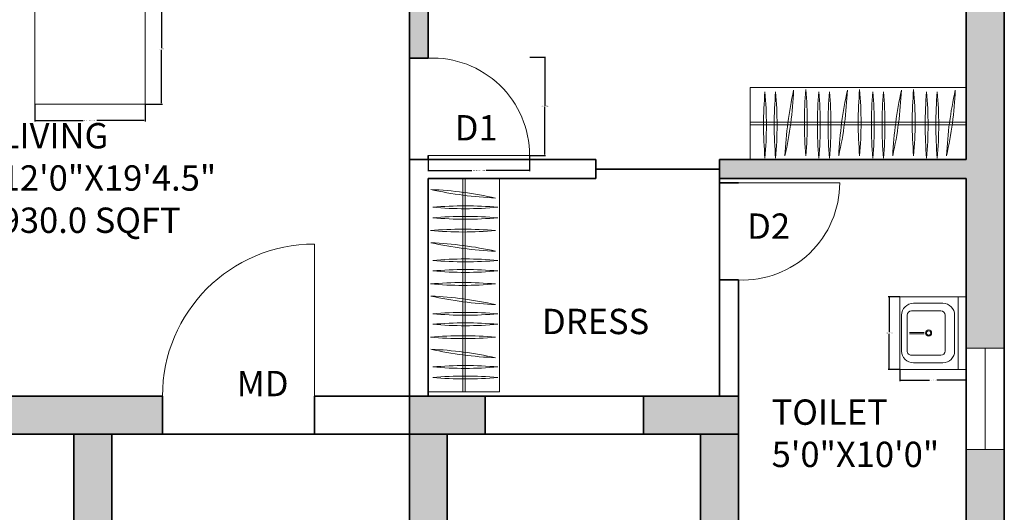
# Model space of a CAD drawing. Units: inches. Extents: x -9 to 505, y -680 to 48.
# Tile 7 of 17: x 235 to 469, y -314 to -198. Entities that reach past the tile are written whole.
import ezdxf

# ---------------------------------------------------------------- set-up
doc = ezdxf.new("R2010")
doc.units = ezdxf.units.IN
doc.header["$MEASUREMENT"] = 0
for name, color, linetype, lineweight in [('A-ANNO-DIMS', 2, 'Continuous', 18), ('A-ANNO-TEXT', 7, 'Continuous', 18), ('A-AREA-IDEN', 7, 'Continuous', 18), ('A-DOOR', 3, 'Continuous', 18), ('A-FLOR-CASE', 8, 'Continuous', 18), ('A-FLOR-FIXT', 9, 'Continuous', 18), ('A-FURN', 8, 'Continuous', 18), ('A-GLAZ', 4, 'Continuous', 18), ('A-WALL', 7, 'Continuous', 35), ('A-WALL-PATT', 251, 'Continuous', 13), ('S-CONC', 7, 'Continuous', 35), ('S-CONC-PATT', 18, 'Continuous', 13)]:
    doc.layers.add(name, color=color, linetype=linetype, lineweight=lineweight)
doc.styles.get("Standard").update_dxf_attribs({"font": 'arial.ttf'})
doc.dimstyles.get("Standard").update_dxf_attribs({"dimtxt": 0.18, "dimasz": 0.18, "dimexe": 0.18, "dimexo": 0.0625, "dimgap": 0.09, "dimtad": 0, "dimtih": 1, "dimtoh": 1, "dimdec": 0, "dimzin": 0, "dimdsep": 46, "dimlunit": 3, "dimtxsty": 'Standard', "dimcen": 0.09, "dimadec": 0, "dimazin": 0, "dimtfac": 1, "dimtdec": 0, "dimtofl": 0, "dimtmove": 0, "dimatfit": 3, "dimfxl": 1, "dimtolj": 1, "dimtzin": 0, "dimarcsym": 0})

# ---------------------------------------------------------------- blocks, each defined once
blk = doc.blocks.new('М14 600х655')
for p, q in [((-655, 600), (-655, 0)), ((-655, 600), (-655, 0)), ((-655, 0), (-655, 600)), ((0, 600), (-655, 600)), ((0, 0), (0, 600)), ((0, 525), (-655, 525)), ((-165.1, 494.1), (-489.9, 494.1)), ((-595.8, 388.1), (-595.8, 121.3)), ((-528.4, 370.1), (-528.4, 103.3)), ((-165.4, 408.4), (-490.2, 408.4)), ((-127.2, 103.3), (-127.2, 370.1)), ((-59.2, 121.3), (-59.2, 388.1)), ((-333.5, 87.1), (-333.5, 219.6)), ((-321.5, 87.1), (-321.5, 219.6)), ((-655, 0), (-655, 0)), ((-655, 0), (-655, 0)), ((-655, 0), (0, 0)), ((-655, 0), (0, 0)), ((-490.2, 65.1), (-165.4, 65.1)), ((-489.9, 15.4), (-165.1, 15.4))]:
    blk.add_line(p, q)
for radius in [27.6, 19.3]:
    blk.add_circle((-327.5, 258.9), radius)
for centre, radius, start, end in [((-489.9, 388.1), 105.9, 90, 180), ((-165.1, 388.1), 105.9, 0, 90), ((-490.2, 370.1), 38.2, 90, 180), ((-165.4, 370.1), 38.2, 0, 90), ((-489.9, 121.3), 105.9, 180, 270), ((-490.2, 103.3), 38.2, 180, 270), ((-165.4, 103.3), 38.2, 270, 0), ((-165.1, 121.3), 105.9, 270, 0)]:
    blk.add_arc(centre, radius, start, end)
blk = doc.blocks.new('WARDROBE-HANGING')
for p, q in [((51.19, 17.07), (0, 17.07)), ((0, 17.07), (0, 0)), ((51.19, 17.07), (51.19, 0)), ((51.19, 8.82), (0, 8.82)), ((51.19, 8.25), (0, 8.25)), ((51.19, 0), (0, 0))]:
    blk.add_line(p, q)
for centre, start, end in [((-79.45, 20.34), 347.508, 357.5023), ((97.92, -3), 167.508, 177.5023), ((102.6, 8.74), 175.0028, 184.9972), ((-76.3, 8.74), 355.0028, 4.9972), ((-66.7, 20.34), 347.508, 357.5023), ((110.67, -3), 167.508, 177.5023), ((115.36, 8.74), 175.0028, 184.9972), ((-63.54, 8.74), 355.0028, 4.9972), ((123.47, -3), 167.508, 177.5023), ((-53.9, 20.34), 347.508, 357.5023), ((128.16, 8.74), 175.0028, 184.9972), ((-50.74, 8.74), 355.0028, 4.9972), ((136.23, -3), 167.508, 177.5023), ((-41.14, 20.34), 347.508, 357.5023), ((92.92, 8.19), 175.0028, 184.9972), ((-85.98, 8.19), 355.0028, 4.9972), ((95.45, 8.19), 175.0028, 184.9972), ((-83.45, 8.19), 355.0028, 4.9972), ((105.68, 8.19), 175.0028, 184.9972), ((-73.22, 8.19), 355.0028, 4.9972), ((108.21, 8.19), 175.0028, 184.9972), ((-70.69, 8.19), 355.0028, 4.9972), ((118.48, 8.19), 175.0028, 184.9972), ((-60.42, 8.19), 355.0028, 4.9972), ((121.01, 8.19), 175.0028, 184.9972), ((-57.89, 8.19), 355.0028, 4.9972), ((131.23, 8.19), 175.0028, 184.9972), ((-47.67, 8.19), 355.0028, 4.9972), ((133.76, 8.19), 175.0028, 184.9972), ((-45.14, 8.19), 355.0028, 4.9972)]:
    blk.add_arc(centre, 89.79, start, end)
blk = doc.blocks.new('WIN-24')
for p, q in [((0, 24), (0, 0)), ((9, 24), (0, 24)), ((4.5, 24), (4.5, 2.23)), ((9, 0), (9, 24)), ((0, 0), (9, 0)), ((4.5, 2.23), (4.5, 0))]:
    blk.add_line(p, q)
blk = doc.blocks.new('DOOR-SWING-24')
blk.add_line((0, 0), (24, 0))
blk.add_arc((0.98, 0), 23.02, 0, 92.4378)
blk = doc.blocks.new('DOOR-ENTRY-36')
blk.add_line((36, 0), (36, 36))
blk.add_arc((36, 0), 36, 90, 180)
blk = doc.blocks.new('TABLE-COFFEE-SQUARE')
at = {"ltscale": 0.03}
blk.add_lwpolyline([(0, 0), (26.11, 0), (26.11, 26.11), (0, 26.11)], close=True, dxfattribs=at)
blk = doc.blocks.new('*D24')
at = {"layer": 'A-ANNO-DIMS', "color": 0, "lineweight": -2, "transparency": 16777216}
for p, q in [((332.26, -230.06), (332.26, -233.78)), ((356.26, -230.06), (356.26, -233.78)), ((332.44, -233.6), (342.58, -233.6)), ((356.08, -233.6), (345.94, -233.6))]:
    blk.add_line(p, q, dxfattribs=at)
at = {"layer": 'A-ANNO-DIMS', "color": 0, "transparency": 16777216}
for points in [[(332.44, -233.57), (332.44, -233.63), (332.26, -233.6)], [(356.08, -233.57), (356.08, -233.63), (356.26, -233.6)]]:
    blk.add_solid(points, dxfattribs=at)
at = {"layer": 'Defpoints', "color": 0, "transparency": 16777216}
for p in [(332.26, -230), (356.26, -230), (356.26, -233.6)]:
    blk.add_point(p, dxfattribs=at)
at = {"layer": 'A-ANNO-DIMS', "color": 0, "transparency": 16777216, "insert": (344.26, -233.6), "char_height": 0.18, "attachment_point": 5}
blk.add_mtext('\\A1;INTERIOR DOOR 2\'-0" TYP.', dxfattribs=at)
blk = doc.blocks.new('*D25')
at = {"layer": 'A-ANNO-DIMS', "color": 0, "lineweight": -2, "transparency": 16777216}
for p, q in [((356.33, -206.73), (360.04, -206.73)), ((359.86, -206.91), (359.86, -218.18)), ((359.86, -229.82), (359.86, -218.55)), ((356.33, -230), (360.04, -230))]:
    blk.add_line(p, q, dxfattribs=at)
at = {"layer": 'A-ANNO-DIMS', "color": 0, "transparency": 16777216}
for points in [[(359.83, -206.91), (359.89, -206.91), (359.86, -206.73)], [(359.83, -229.82), (359.89, -229.82), (359.86, -230)]]:
    blk.add_solid(points, dxfattribs=at)
at = {"layer": 'Defpoints', "color": 0, "transparency": 16777216}
for p in [(356.26, -206.73), (359.86, -206.73), (356.26, -230)]:
    blk.add_point(p, dxfattribs=at)
at = {"layer": 'A-ANNO-DIMS', "color": 0, "transparency": 16777216, "insert": (359.86, -218.37), "char_height": 0.18, "attachment_point": 5}
blk.add_mtext('\\A1;1\'-11 1/2" TYP.', dxfattribs=at)
blk = doc.blocks.new('*D36')
at = {"layer": 'A-ANNO-DIMS', "color": 0, "lineweight": -2, "transparency": 16777216}
for p, q in [((443.97, -263.48), (441.27, -263.48)), ((441.45, -263.66), (441.45, -271.88)), ((441.45, -280.47), (441.45, -272.25)), ((443.97, -280.65), (441.27, -280.65))]:
    blk.add_line(p, q, dxfattribs=at)
at = {"layer": 'A-ANNO-DIMS', "color": 0, "transparency": 16777216}
for points in [[(441.42, -263.66), (441.48, -263.66), (441.45, -263.48)], [(441.42, -280.47), (441.48, -280.47), (441.45, -280.65)]]:
    blk.add_solid(points, dxfattribs=at)
at = {"layer": 'Defpoints', "color": 0, "transparency": 16777216}
for p in [(444.03, -263.48), (441.45, -280.65), (444.03, -280.65)]:
    blk.add_point(p, dxfattribs=at)
at = {"layer": 'A-ANNO-DIMS', "color": 0, "transparency": 16777216, "insert": (441.45, -272.06), "char_height": 0.18, "attachment_point": 5}
blk.add_mtext('\\A1;BASIN 1\'-5" TYP.', dxfattribs=at)
blk = doc.blocks.new('*D37')
at = {"layer": 'A-ANNO-DIMS', "color": 0, "lineweight": -2, "transparency": 16777216}
for p, q in [((444.03, -280.71), (444.03, -283.41)), ((459.76, -280.71), (459.76, -283.41)), ((444.21, -283.23), (451.06, -283.23)), ((459.58, -283.23), (452.74, -283.23))]:
    blk.add_line(p, q, dxfattribs=at)
at = {"layer": 'A-ANNO-DIMS', "color": 0, "transparency": 16777216}
for points in [[(444.21, -283.2), (444.21, -283.26), (444.03, -283.23)], [(459.58, -283.2), (459.58, -283.26), (459.76, -283.23)]]:
    blk.add_solid(points, dxfattribs=at)
at = {"layer": 'Defpoints', "color": 0, "transparency": 16777216}
for p in [(444.03, -280.65), (459.76, -280.65), (459.76, -283.23)]:
    blk.add_point(p, dxfattribs=at)
at = {"layer": 'A-ANNO-DIMS', "color": 0, "transparency": 16777216, "insert": (451.9, -283.23), "char_height": 0.18, "attachment_point": 5}
blk.add_mtext('\\A1;1\'-3 1/2" TYP.', dxfattribs=at)
blk = doc.blocks.new('*D38')
at = {"layer": 'A-ANNO-DIMS', "color": 0, "lineweight": -2, "transparency": 16777216}
for p, q in [((239.02, -217.94), (239.02, -221.97)), ((265.13, -217.94), (265.13, -221.97)), ((239.2, -221.79), (250.46, -221.79)), ((264.95, -221.79), (253.7, -221.79))]:
    blk.add_line(p, q, dxfattribs=at)
at = {"layer": 'A-ANNO-DIMS', "color": 0, "transparency": 16777216}
for points in [[(239.2, -221.76), (239.2, -221.82), (239.02, -221.79)], [(264.95, -221.76), (264.95, -221.82), (265.13, -221.79)]]:
    blk.add_solid(points, dxfattribs=at)
at = {"layer": 'Defpoints', "color": 0, "transparency": 16777216}
for p in [(239.02, -217.87), (265.13, -217.87), (265.13, -221.79)]:
    blk.add_point(p, dxfattribs=at)
at = {"layer": 'A-ANNO-DIMS', "color": 0, "transparency": 16777216, "insert": (252.08, -221.79), "char_height": 0.18, "attachment_point": 5}
blk.add_mtext('\\A1;COFFEE TABLE 2\'-2" TYP.', dxfattribs=at)
blk = doc.blocks.new('*D39')
at = {"layer": 'A-ANNO-DIMS', "color": 0, "lineweight": -2, "transparency": 16777216}
for p, q in [((265.2, -191.76), (269.23, -191.76)), ((269.05, -191.94), (269.05, -204.64)), ((269.05, -217.69), (269.05, -205)), ((265.2, -217.87), (269.23, -217.87))]:
    blk.add_line(p, q, dxfattribs=at)
at = {"layer": 'A-ANNO-DIMS', "color": 0, "transparency": 16777216}
for points in [[(269.02, -191.94), (269.08, -191.94), (269.05, -191.76)], [(269.02, -217.69), (269.08, -217.69), (269.05, -217.87)]]:
    blk.add_solid(points, dxfattribs=at)
at = {"layer": 'Defpoints', "color": 0, "transparency": 16777216}
for p in [(265.13, -191.76), (269.05, -191.76), (265.13, -217.87)]:
    blk.add_point(p, dxfattribs=at)
at = {"layer": 'A-ANNO-DIMS', "color": 0, "transparency": 16777216, "insert": (269.05, -204.82), "char_height": 0.18, "attachment_point": 5}
blk.add_mtext('\\A1;2\'-2" TYP.', dxfattribs=at)

msp = doc.modelspace()

# ---------------------------------------------------------------- hatches: boundary and pattern name
at = {"layer": 'A-WALL-PATT'}
h = msp.add_hatch(color=256, dxfattribs=at)
h.dxf.hatch_style = 1
h.paths.add_polyline_path([(101.64, 11.5), (48.26, 11.5), (48.26, 2.5), (72.26, 2.5), (72.26, -21.25), (81.26, -21.25), (81.26, 2.5), (101.64, 2.5)])
h.paths.add_polyline_path([(36.26, 2.5), (27.26, 2.5), (27.26, -6.92), (36.26, -6.92)])
h.paths.add_polyline_path([(81.26, -57.25), (72.26, -57.25), (72.26, -75.5), (81.26, -75.5)])
h.paths.add_polyline_path([(162.76, 11.5), (137.64, 11.5), (137.64, 2.5), (162.76, 2.5)])
h.paths.add_polyline_path([(179.26, 2.5), (174.76, 2.5), (174.76, -75.5), (179.26, -75.5), (179.26, -54.5), (229.51, -54.5), (229.51, -45.5), (179.26, -45.5)])
h.paths.add_polyline_path([(382.26, -45.5), (332.26, -45.5), (332.26, 2.5), (327.76, 2.5), (327.76, -45.5), (277.51, -45.5), (277.51, -54.5), (327.76, -54.5), (327.76, -111.5), (332.26, -111.5), (332.26, -54.5), (382.26, -54.5)])
h.paths.add_polyline_path([(332.26, -128), (327.76, -128), (327.76, -207), (332.26, -207)])
h.paths.add_polyline_path([(124.76, -111.5), (36.26, -111.5), (36.26, -116), (120.26, -116), (120.26, -168.5), (179.26, -168.5), (179.26, -164), (124.76, -164)])
h.paths.add_polyline_path([(96.26, -164), (36.26, -164), (36.26, -152), (27.26, -152), (27.26, -208.88), (36.26, -208.88), (36.26, -168.5), (96.26, -168.5)])
h.paths.add_polyline_path([(36.26, -244.88), (27.26, -244.88), (27.26, -287), (36.26, -287)])
h.paths.add_polyline_path([(179.26, -204.5), (174.76, -204.5), (174.76, -287), (179.26, -287)])
h.paths.add_polyline_path([(257.26, -296), (248.26, -296), (248.26, -446), (269.26, -446), (269.26, -437), (257.26, -437)])
h.paths.add_polyline_path([(90.26, -296), (81.26, -296), (81.26, -348.67), (90.26, -348.67)])
h.paths.add_polyline_path([(90.26, -384.67), (81.26, -384.67), (81.26, -416), (90.26, -416)])
h.paths.add_polyline_path([(170.26, -452), (36.26, -452), (36.26, -456.5), (165.76, -456.5), (165.76, -504.5), (165.13, -504.5), (165.13, -509), (170.26, -509)])
h.paths.add_polyline_path([(141.76, -504.5), (36.26, -504.5), (36.26, -492.5), (27.26, -492.5), (27.26, -565.96), (36.26, -565.96), (36.26, -509), (141.76, -509)])
h.paths.add_polyline_path([(36.26, -601.96), (27.26, -601.96), (27.26, -658.5), (36.26, -658.5)])
h.paths.add_polyline_path([(170.26, -670.5), (170.26, -634.5), (222.76, -634.5), (222.76, -625.5), (165.76, -625.5), (165.76, -670.5), (36.26, -670.5), (36.26, -679.5), (170.26, -679.5)])
h.paths.add_polyline_path([(332.26, -616.5), (433.89, -616.5), (433.89, -612), (332.26, -612), (332.26, -610.56), (327.76, -610.56), (327.76, -625.5), (270.76, -625.5), (270.76, -634.5), (327.76, -634.5), (327.76, -658.5), (332.26, -658.5)])
h.paths.add_polyline_path([(459.76, -670.5), (336.76, -670.5), (336.76, -679.5), (459.76, -679.5)])
h.paths.add_polyline_path([(468.76, -545.74), (459.76, -545.74), (459.76, -612), (457.89, -612), (457.89, -616.5), (459.76, -616.5), (459.76, -658.5), (468.76, -658.5)])
h.paths.add_polyline_path([(332.26, -446), (327.76, -446), (327.76, -574.56), (332.26, -574.56)])
h.paths.add_polyline_path([(327.76, -437), (305.26, -437), (305.26, -446), (327.76, -446)])
h.paths.add_polyline_path([(459.76, -437), (348.76, -437), (348.76, -446), (459.76, -446)])
h.paths.add_polyline_path([(468.76, -458), (459.76, -458), (459.76, -509.74), (468.76, -509.74)])
h.paths.add_polyline_path([(468.76, -365), (459.76, -365), (459.76, -437), (468.76, -437)])
h.paths.add_polyline_path([(468.76, -299.6), (459.76, -299.6), (459.76, -344), (468.76, -344)])
h.paths.add_polyline_path([(468.76, -184.74), (459.76, -184.74), (459.76, -231), (401.26, -231), (401.26, -235.5), (459.76, -235.5), (459.76, -275.6), (468.76, -275.6)])
h.paths.add_polyline_path([(390.76, -356), (342.76, -356), (342.76, -365), (390.76, -365)])
h.paths.add_polyline_path([(459.76, -356), (405.76, -356), (405.76, -365), (459.76, -365)])
h.paths.add_polyline_path([(405.76, -296), (396.76, -296), (396.76, -356), (405.76, -356)])
h.paths.add_polyline_path([(336.76, -296), (327.76, -296), (327.76, -356), (336.76, -356)])
h.paths.add_polyline_path([(468.76, -9.5), (459.76, -9.5), (459.76, -45.5), (418.26, -45.5), (418.26, -54.5), (468.76, -54.5)])
h.paths.add_polyline_path([(468.76, -54.5), (459.76, -54.5), (459.76, -111.5), (468.76, -111.5)])
h.paths.add_polyline_path([(468.76, -128), (459.76, -128), (459.76, -148.74), (468.76, -148.74)])
at = {"layer": 'S-CONC-PATT'}
h = msp.add_hatch(color=256, dxfattribs=at)
h.dxf.hatch_style = 1
h.paths.add_polyline_path([(269.26, -296), (269.26, -287), (27.26, -287), (27.26, -308), (36.26, -308), (36.26, -296)])
h = msp.add_hatch(color=256, dxfattribs=at)
h.dxf.hatch_style = 1
h.paths.add_polyline_path([(345.76, -287), (327.76, -287), (327.76, -296), (345.76, -296)])
h.paths.add_polyline_path([(405.76, -287), (383.26, -287), (383.26, -296), (405.76, -296)])

# ---------------------------------------------------------------- linework, layer by layer
at = {"layer": 'A-FLOR-CASE'}
for p, q in [((332.26, -235.5), (332.26, -286)), ((332.26, -235.5), (349.1, -235.5)), ((340.4, -235.5), (340.4, -286)), ((340.96, -235.5), (340.96, -286)), ((349.1, -235.5), (349.1, -286)), ((332.26, -286), (349.1, -286))]:
    msp.add_line(p, q, dxfattribs=at)
for centre, start, end in [((352.05, -151.61), 257.508, 267.5023), ((329.03, -326.59), 77.508, 87.5023), ((341.02, -330.53), 85.0028, 94.9972), ((341.02, -154.05), 265.0028, 274.9972), ((341.02, -333.03), 85.0028, 94.9972), ((341.02, -156.54), 265.0028, 274.9972), ((340.47, -336.06), 85.0028, 94.9972), ((340.47, -159.57), 265.0028, 274.9972), ((352.05, -164.2), 257.508, 267.5023), ((329.03, -339.17), 77.508, 87.5023), ((341.02, -343.11), 85.0028, 94.9972), ((341.02, -166.63), 265.0028, 274.9972), ((341.02, -345.61), 85.0028, 94.9972), ((341.02, -169.12), 265.0028, 274.9972), ((340.47, -348.69), 85.0028, 94.9972), ((340.47, -172.2), 265.0028, 274.9972), ((329.03, -351.8), 77.508, 87.5023), ((352.05, -176.83), 257.508, 267.5023), ((341.02, -355.74), 85.0028, 94.9972), ((341.02, -179.26), 265.0028, 274.9972), ((341.02, -358.24), 85.0028, 94.9972), ((341.02, -181.75), 265.0028, 274.9972), ((340.47, -361.27), 85.0028, 94.9972), ((340.47, -184.79), 265.0028, 274.9972), ((329.03, -364.39), 77.508, 87.5023), ((352.05, -189.41), 257.508, 267.5023), ((341.02, -368.33), 85.0028, 94.9972), ((341.02, -191.84), 265.0028, 274.9972), ((341.02, -370.82), 85.0028, 94.9972), ((341.02, -194.34), 265.0028, 274.9972)]:
    msp.add_arc(centre, 88.58, start, end, dxfattribs=at)
at = {"layer": 'A-WALL'}
for p, q in [((468.76, 11.5), (468.76, -679.5)), ((327.76, -54.5), (327.76, -287)), ((332.26, -54.5), (332.26, -207)), ((459.76, -54.5), (459.76, -231)), ((332.26, -207), (327.76, -207)), ((332.26, -231), (327.76, -231)), ((332.26, -230), (332.26, -231)), ((332.26, -231), (371.97, -231)), ((371.97, -231), (371.97, -235.5)), ((401.26, -231), (401.26, -287)), ((401.26, -231), (459.76, -231)), ((371.97, -233.25), (401.26, -233.25)), ((332.26, -235.5), (371.97, -235.5)), ((332.26, -235.5), (332.26, -287)), ((401.26, -235.5), (459.76, -235.5)), ((459.76, -235.5), (459.76, -612)), ((401.26, -236.5), (405.76, -236.5)), ((401.26, -259.5), (405.76, -259.5)), ((405.76, -259.5), (405.76, -356)), ((305.26, -287), (305.26, -296)), ((305.26, -287), (405.76, -287)), ((36.26, -296), (405.76, -296)), ((248.26, -296), (248.26, -446)), ((257.26, -296), (257.26, -437)), ((327.76, -296), (327.76, -365)), ((336.76, -296), (336.76, -356)), ((396.76, -296), (396.76, -356))]:
    msp.add_line(p, q, dxfattribs=at)
at = {"layer": 'S-CONC'}
for p, q in [((27.26, -287), (269.26, -287)), ((269.26, -296), (269.26, -287)), ((327.76, -296), (327.76, -287)), ((345.76, -287), (345.76, -296)), ((383.26, -287), (383.26, -296))]:
    msp.add_line(p, q, dxfattribs=at)

# ---------------------------------------------------------------- block references
at = {"layer": 'A-DOOR'}
for name, p in [('DOOR-SWING-24', (332.26, -230)), ('DOOR-ENTRY-36', (269.26, -287))]:
    msp.add_blockref(name, p, dxfattribs=at)
at = {"layer": 'A-DOOR', "extrusion": (0, 0, -1), "zscale": -1, "rotation": 180}
msp.add_blockref('DOOR-SWING-24', (-405.76, -236.5), dxfattribs=at)
at = {"layer": 'A-FLOR-CASE'}
msp.add_blockref('WARDROBE-HANGING', (408.57, -231), dxfattribs=at)
at = {"layer": 'A-FLOR-FIXT', "xscale": 0.0262208519320216, "yscale": 0.0262208519320216, "zscale": 0.0262208519320216, "rotation": 270}
msp.add_blockref('М14 600х655', (444.03, -280.65), dxfattribs=at)
at = {"layer": 'A-FURN'}
msp.add_blockref('TABLE-COFFEE-SQUARE', (239.02, -217.87), dxfattribs=at)
at = {"layer": 'A-GLAZ'}
msp.add_blockref('WIN-24', (459.76, -299.6), dxfattribs=at)

# ---------------------------------------------------------------- texts
at = {"layer": 'A-ANNO-TEXT', "char_height": 6, "attachment_point": 1}
for s, insert in [('D1', (338.52, -220.48)), ('D2', (407.82, -243.76))]:
    msp.add_mtext(s, dxfattribs=dict(at, insert=insert))
at = {"layer": 'A-ANNO-TEXT', "insert": (286.86, -281.02), "char_height": 6, "attachment_point": 1}
msp.add_mtext_dynamic_manual_height_columns('MD', width=0.5067, gutter_width=1, heights=[0], dxfattribs=at)
at = {"layer": 'A-AREA-IDEN', "char_height": 6, "attachment_point": 1}
for s, insert in [('LIVING\\P12\'0"X19\'4.5"\\P930.0 SQFT', (230.92, -222.36)), ('DRESS', (359.2, -266.32)), ('TOILET\\P5\'0"X10\'0"', (413.62, -287.78))]:
    msp.add_mtext(s, dxfattribs=dict(at, insert=insert))

# ---------------------------------------------------------------- dimensions: what is measured, and where the dimension line sits
at = {"layer": 'A-ANNO-DIMS'}
for base, p1, p2, angle, text, picture, middle in [((269.05, -191.76), (265.13, -217.87), (265.13, -191.76), 90, '<> TYP.', '*D39', (269.05, -204.82)), ((359.86, -206.73), (356.26, -230), (356.26, -206.73), 90, '<> TYP.', '*D25', (359.86, -218.37)), ((441.45, -280.65), (444.03, -263.48), (444.03, -280.65), 270, 'BASIN <> TYP.', '*D36', (441.45, -272.06))]:
    dim = msp.add_linear_dim(base=base, p1=p1, p2=p2, angle=angle, text=text, dimstyle='Standard', override={"dimdec": 1, "dimlfac": 1, "dimrnd": 0, "dimzin": 1, "dimdsep": 46, "dimlunit": 4, "dimfrac": 2}, dxfattribs=at)
    dim.commit()
    dim.dimension.update_dxf_attribs({"geometry": picture, "text_midpoint": middle})
for base, p1, p2, text, picture, middle in [((265.13, -221.79), (239.02, -217.87), (265.13, -217.87), 'COFFEE TABLE <> TYP.', '*D38', (252.08, -221.79)), ((356.26, -233.6), (332.26, -230), (356.26, -230), 'INTERIOR DOOR <> TYP.', '*D24', (344.26, -233.6)), ((459.76, -283.23), (444.03, -280.65), (459.76, -280.65), '<> TYP.', '*D37', (451.9, -283.23))]:
    dim = msp.add_linear_dim(base=base, p1=p1, p2=p2, text=text, dimstyle='Standard', override={"dimdec": 1, "dimlfac": 1, "dimrnd": 0, "dimzin": 1, "dimdsep": 46, "dimlunit": 4, "dimfrac": 2}, dxfattribs=at)
    dim.commit()
    dim.dimension.update_dxf_attribs({"geometry": picture, "text_midpoint": middle})

doc.saveas('drawing.dxf')
